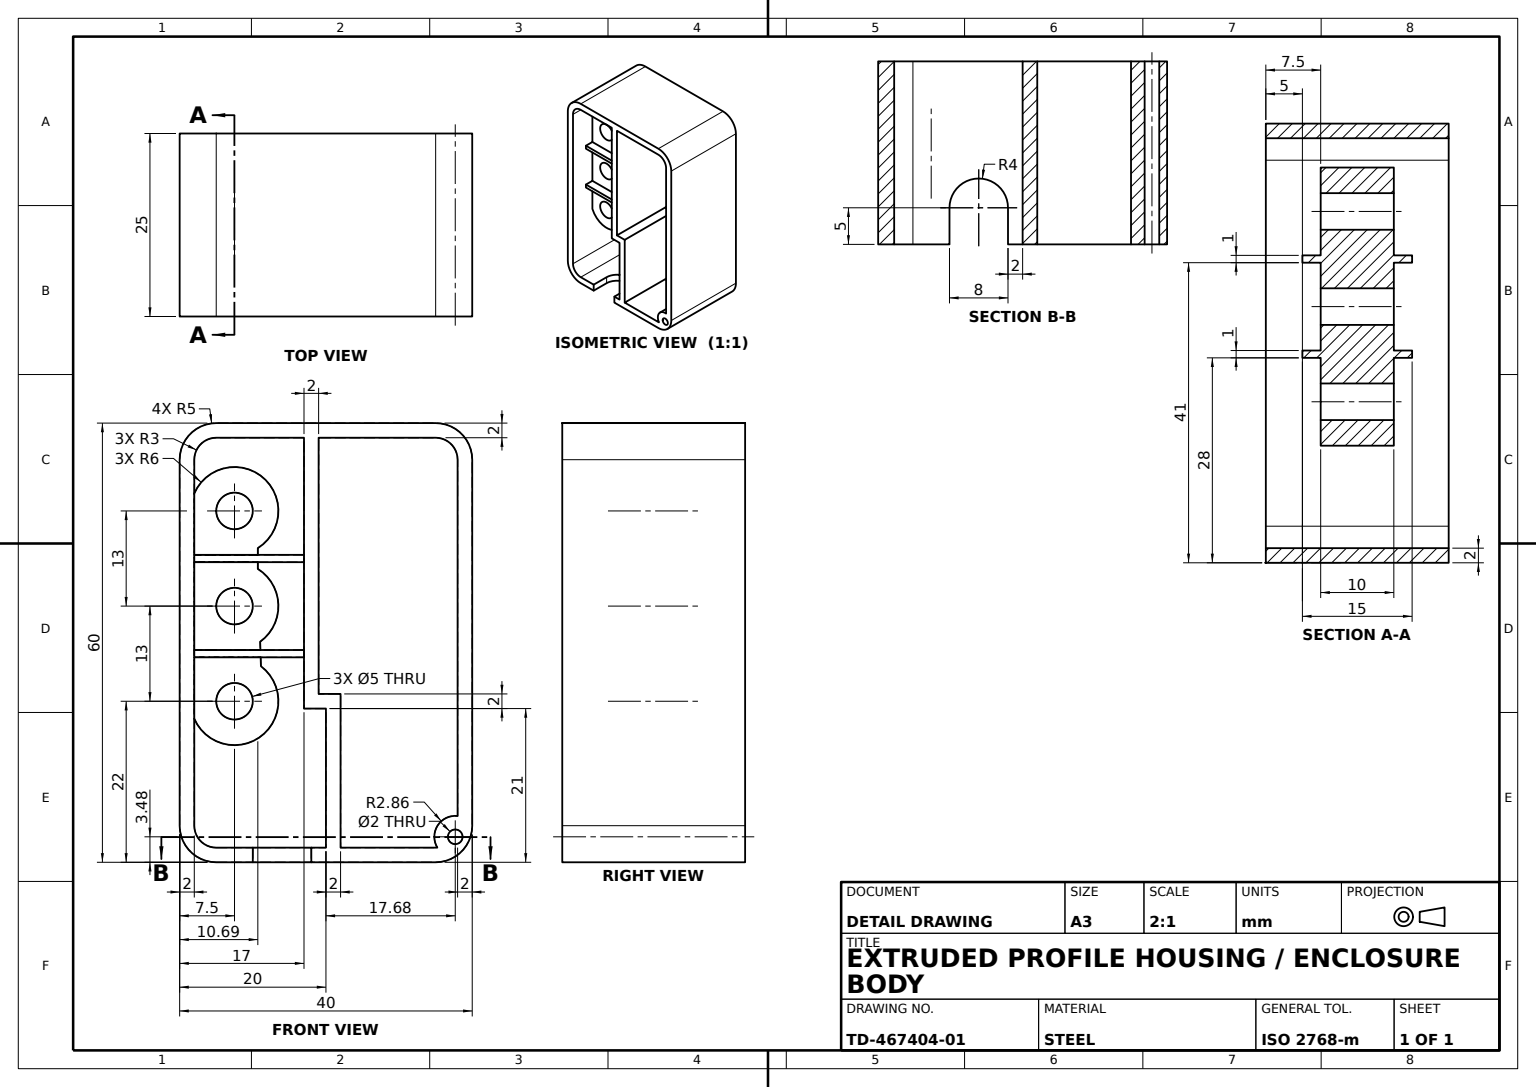
from build123d import *

# Parameters (mm, degrees)
BOX_PROFILE_SKETCH_R      = 1
BOX_SHELL_25MM_DEPTH      = 12.5
PARTITION_WALL_15MM_DEPTH = 7.5
SKETCH1_5_R               = 2.5
PARTITION_WALL_10MM_DEPTH = 5
NOTCH_CUT_4MM_DEPTH       = 65.468984791
NOTCH_CUT_4MM_DEPTH_BACK  = 4


with BuildPart() as part:
    # Box Profile Sketch → Box Shell 25mm (new, symmetric)
    with BuildSketch(Plane.XY):
        with BuildLine():
            Line((15, 30), (-15, 30))
            ThreePointArc((-15, 30), (-18.535533906, 28.535533906), (-20, 25))
            Line((-20, 25), (-20, -25))
            ThreePointArc((-20, -25), (-18.535533906, -28.535533906), (-15, -30))
            Line((-15, -30), (-7, -30))
            Line((-7, -30), (-3, -30))
            Line((-3, -30), (15, -30))
            ThreePointArc((15, -30), (18.535533906, -28.535533906), (20, -25))
            Line((20, -25), (20, 25))
            ThreePointArc((20, 25), (18.535533906, 28.535533906), (15, 30))
        make_face()
        with BuildLine():
            ThreePointArc((-18, 25), (-17.121320344, 27.121320344), (-15, 28))
            Line((-15, 28), (-3, 28))
            Line((-3, 28), (-3, 11.9990204))
            Line((-3, 11.9990204), (-3, 10.9990204))
            Line((-3, 10.9990204), (-3, -1.0009796))
            Line((-3, -1.0009796), (-3, -2.0009796))
            Line((-3, -2.0009796), (-3, -9))
            Line((-3, -9), (0, -9))
            Line((0, -9), (0, -28))
            Line((0, -28), (-3, -28))
            Line((-3, -28), (-7, -28))
            Line((-7, -28), (-15, -28))
            ThreePointArc((-15, -28), (-17.121320344, -27.121320344), (-18, -25))
            Line((-18, -25), (-18, -10.398895362))
            Line((-18, -10.398895362), (-18, -2.0009796))
            Line((-18, -2.0009796), (-18, -1.0009796))
            Line((-18, -1.0009796), (-18, 10.9990204))
            Line((-18, 10.9990204), (-18, 11.9990204))
            Line((-18, 11.9990204), (-18, 20.396936162))
            Line((-18, 20.396936162), (-18, 25))
        make_face(mode=Mode.SUBTRACT)
        with Locations((17.67963323, -26.519449845)):
            Circle(BOX_PROFILE_SKETCH_R, mode=Mode.SUBTRACT)
        with BuildLine():
            ThreePointArc((15, 28), (17.121320344, 27.121320344), (18, 25))
            Line((18, 25), (18, -23.676308898))
            ThreePointArc((18, -23.676308898), (15.270156966, -24.976559879), (15.23135699, -28))
            Line((15.23135699, -28), (2, -28))
            Line((2, -28), (2, -7))
            Line((2, -7), (-1, -7))
            Line((-1, -7), (-1, 28))
            Line((-1, 28), (15, 28))
        make_face(mode=Mode.SUBTRACT)
    extrude(amount=BOX_SHELL_25MM_DEPTH, both=True)

    # Sketch1_3 → Partition Wall 15mm (add, symmetric)
    with BuildSketch(Plane.XY):
        Polygon((-3, -2.0009796), (-3, -1.0009796), (-8.958312837, -1.0009796), (-18, -1.0009796), (-18, -2.0009796), (-8.925986332, -2.0009796), align=None)
        Polygon((-3, 10.9990204), (-3, 11.9990204), (-9.312399857, 11.9990204), (-18, 11.9990204), (-18, 10.9990204), (-9.312399857, 10.9990204), align=None)
    extrude(amount=PARTITION_WALL_15MM_DEPTH, both=True)

    # Sketch1_5 → Partition Wall 10mm (add, symmetric)
    # profile 1 of 3: a face of its own
    with BuildSketch(Plane.XY):
        with BuildLine():
            ThreePointArc((-9.312399857, 12.915792555), (-8.584814731, 22.545593209), (-18, 20.396936162))
            Line((-18, 20.396936162), (-18, 11.9990204))
            Line((-18, 11.9990204), (-9.312399857, 11.9990204))
            Line((-9.312399857, 11.9990204), (-9.312399857, 12.915792555))
        make_face()
        with Locations((-12.5, 17.9990204)):
            Circle(SKETCH1_5_R, mode=Mode.SUBTRACT)
    # profile 2 of 3: a face of its own
    with BuildSketch(Plane.XY):
        with BuildLine():
            Line((-9.312399857, 10.082248245), (-9.312399857, 10.9990204))
            Line((-9.312399857, 10.9990204), (-18, 10.9990204))
            Line((-18, 10.9990204), (-18, -1.0009796))
            Line((-18, -1.0009796), (-8.958312837, -1.0009796))
            Line((-8.958312837, -1.0009796), (-8.994851629, 0.129324835))
            ThreePointArc((-8.994851629, 0.129324835), (-6.503051462, 5.190353168), (-9.312399857, 10.082248245))
        make_face()
        with Locations((-12.5, 4.9990204)):
            Circle(SKETCH1_5_R, mode=Mode.SUBTRACT)
    # profile 3 of 3: a face of its own
    with BuildSketch(Plane.XY):
        with BuildLine():
            Line((-8.886875414, -3.210851133), (-8.925986332, -2.0009796))
            Line((-8.925986332, -2.0009796), (-18, -2.0009796))
            Line((-18, -2.0009796), (-18, -10.398895362))
            ThreePointArc((-18, -10.398895362), (-8.784213453, -12.71191691), (-8.886875414, -3.210851133))
        make_face()
        with Locations((-12.5, -8.0009796)):
            Circle(SKETCH1_5_R, mode=Mode.SUBTRACT)
    extrude(amount=PARTITION_WALL_10MM_DEPTH, both=True)

    # Notch Sketch → Notch Cut 4mm (cut, two sides: drawn at the far end of the back side and taken through both)
    with BuildSketch(Plane.XZ.offset(30).offset(-NOTCH_CUT_4MM_DEPTH_BACK)):
        with BuildLine():
            Line((-2, 7.5), (-2, 12.5))
            Line((-2, 12.5), (-10, 12.5))
            Line((-10, 12.5), (-10, 7.5))
            ThreePointArc((-10, 7.5), (-6, 3.5), (-2, 7.5))
        make_face()
    extrude(amount=NOTCH_CUT_4MM_DEPTH + NOTCH_CUT_4MM_DEPTH_BACK, mode=Mode.SUBTRACT)


solid = part.part
